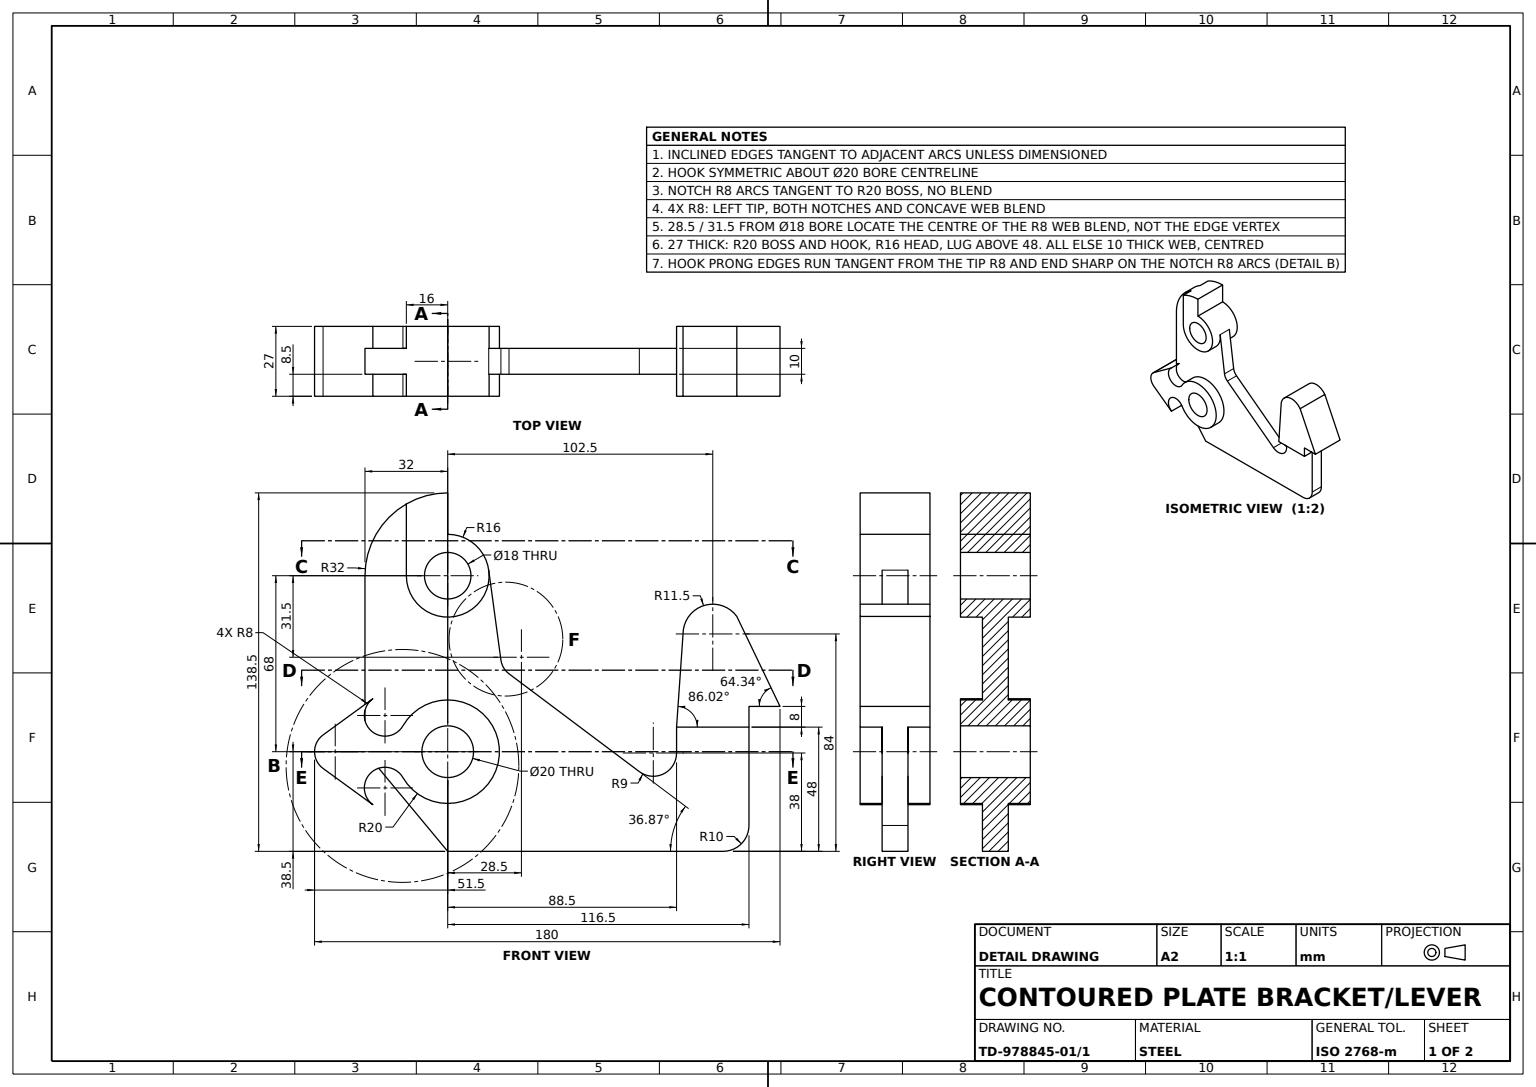
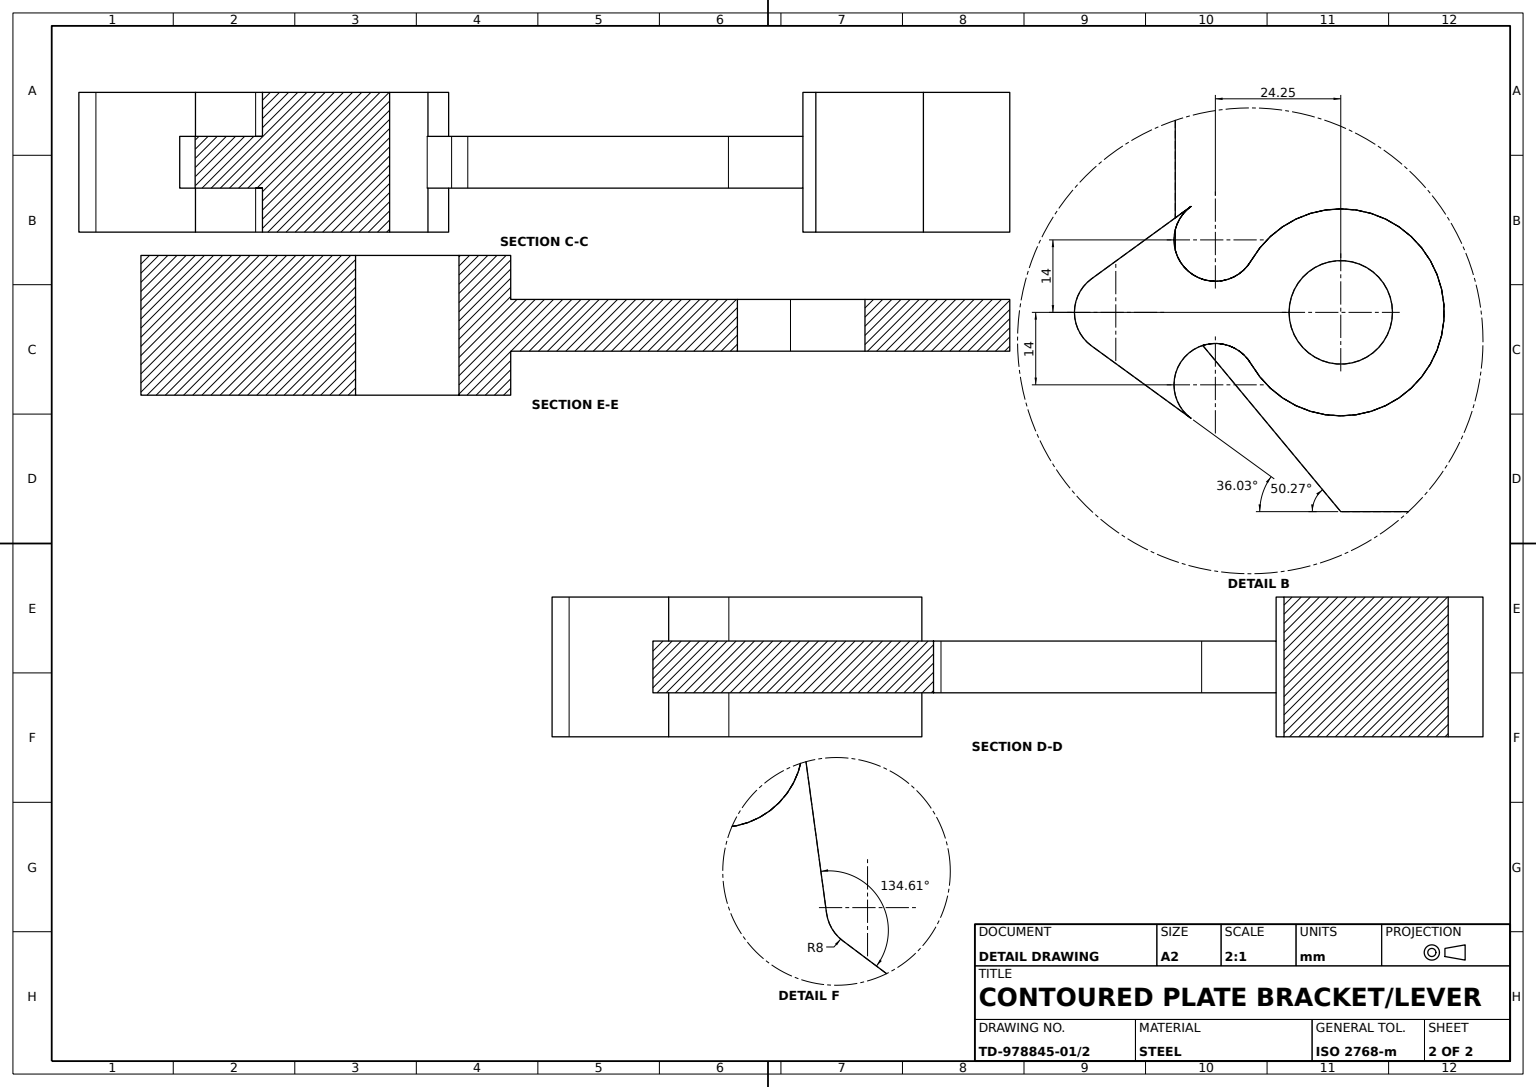
from build123d import *

# Parameters (mm, degrees)
BRACKET_PLATE_DEPTH        = 10
UPPER_PIVOT_BOSS_DEPTH     = 13.5
UPPER_PIVOT_BORE_PROFILE_R = 9
UPPER_PIVOT_BORE_18_DEPTH  = 27
LOWER_PIVOT_BOSS_DEPTH     = 13.5
LOWER_PIVOT_BORE_PROFILE_R = 10
LOWER_PIVOT_BORE_20_DEPTH  = 27
STOP_LUG_DEPTH             = 13.5
PLATE_FILLET_R10_R         = 10


with BuildPart() as part:
    # Bracket Plate Profile → Bracket Plate (new body)
    with BuildSketch(Plane.XY):
        with BuildLine():
            Line((-32, 0), (-32, -68))
            Line((-32, -68), (0, -106.5))
            Line((0, -106.5), (116.5, -106.5))
            Line((116.5, -106.5), (116.5, -58.5))
            Line((116.5, -58.5), (88.5, -58.5))
            Line((88.5, -58.5), (88.5, -68.5))
            ThreePointArc((88.5, -68.5), (83.524922359, -76.549844719), (74.1, -75.7))
            Line((74.1, -75.7), (23.7, -37.9))
            ThreePointArc((23.7, -37.9), (21.602252409, -35.552292952), (20.572822936, -32.576969725))
            Line((20.572822936, -32.576969725), (15.854354129, 2.15393945))
            ThreePointArc((15.854354129, 2.15393945), (10.524660774, 12.051203907), (0, 16))
            Line((0, 16), (0, 32))
            ThreePointArc((0, 32), (-22.627416998, 22.627416998), (-32, 0))
        make_face()
    extrude(amount=BRACKET_PLATE_DEPTH)

    # Upper Pivot Boss Profile → Upper Pivot Boss (add, symmetric)
    with BuildSketch(Plane.XY.offset(5)):
        with BuildLine():
            Line((0, 16), (0, 32))
            ThreePointArc((0, 32), (-8.282209443, 30.909626441), (-16, 27.712812921))
            Line((-16, 27.712812921), (-16, 0))
            ThreePointArc((-16, 0), (11.313708499, -11.313708499), (0, 16))
        make_face()
    extrude(amount=UPPER_PIVOT_BOSS_DEPTH, both=True)

    # Upper Pivot Bore Profile → Upper Pivot Bore Ø18 (cut)
    with BuildSketch(Plane.XY.offset(18.5)):
        Circle(UPPER_PIVOT_BORE_PROFILE_R)
    extrude(amount=-UPPER_PIVOT_BORE_18_DEPTH, mode=Mode.SUBTRACT)

    # Lower Pivot Boss Profile → Lower Pivot Boss (add, symmetric)
    with BuildSketch(Plane.XY.offset(5)):
        with BuildLine():
            Line((-48.20516756, -74.470038503), (-28.953878866, -88.470038503))
            ThreePointArc((-28.953878866, -88.470038503), (-29.600430512, -76.053648048), (-17.320508076, -78))
            ThreePointArc((-17.320508076, -78), (20, -68), (-17.320508076, -58))
            ThreePointArc((-17.320508076, -58), (-29.600430512, -59.946351952), (-28.953878866, -47.529961497))
            Line((-28.953878866, -47.529961497), (-48.20516756, -61.529961497))
            ThreePointArc((-48.20516756, -61.529961497), (-51.5, -68), (-48.20516756, -74.470038503))
        make_face()
    extrude(amount=LOWER_PIVOT_BOSS_DEPTH, both=True)

    # Lower Pivot Bore Profile → Lower Pivot Bore Ø20 (cut)
    with BuildSketch(Plane.XY.offset(18.5)):
        with Locations((0, -68)):
            Circle(LOWER_PIVOT_BORE_PROFILE_R)
    extrude(amount=-LOWER_PIVOT_BORE_20_DEPTH, mode=Mode.SUBTRACT)

    # Stop Lug Profile → Stop Lug (add, symmetric)
    with BuildSketch(Plane.XY.offset(5)):
        with BuildLine():
            Line((116.5, -58.5), (116.5, -50.5))
            Line((116.5, -50.5), (128.5, -50.5))
            Line((128.5, -50.5), (111.797390872, -15.731800611))
            ThreePointArc((111.797390872, -15.731800611), (98.941207721, -11.564507441), (91, -22.5))
            Line((91, -22.5), (88.5, -58.5))
            Line((88.5, -58.5), (116.5, -58.5))
        make_face()
    extrude(amount=STOP_LUG_DEPTH, both=True)

    # Plate Fillet R10
    plate_fillet_r10_edges = [part.edges().sort_by_distance(p)[0] for p in [
        (116.5, -106.5, 5),
    ]]
    fillet(plate_fillet_r10_edges, radius=PLATE_FILLET_R10_R)


solid = part.part
